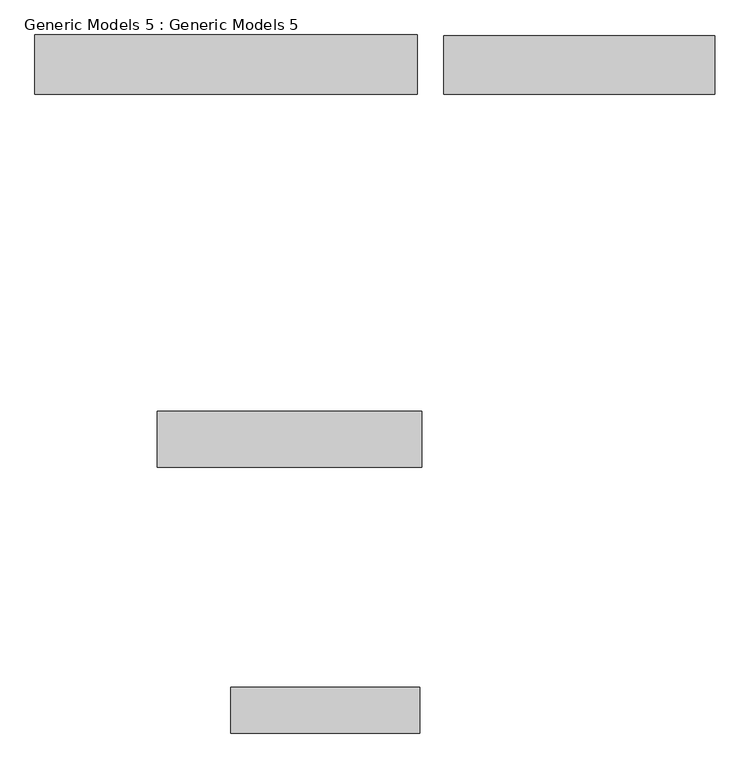
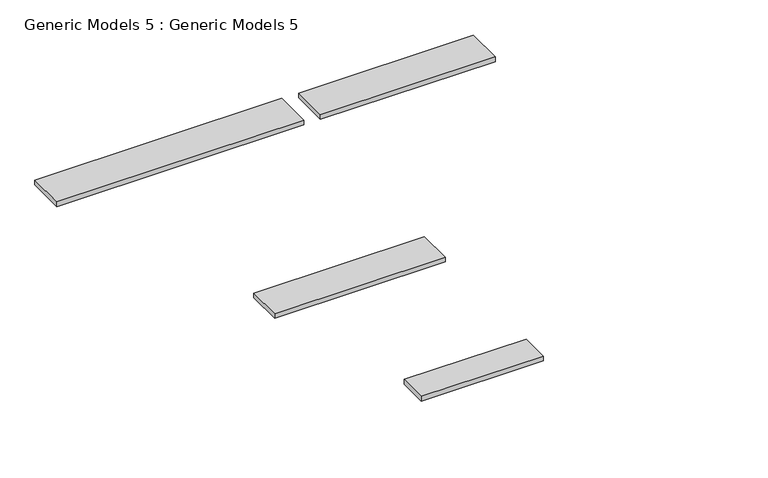
"""IFC4 building model written with IfcOpenShell, lengths in millimetres: proxy geometry, Generic Models 5 : Generic Models 5."""

from ifc_helpers import new_model, si_unit, frame, origin, place, context, project, spatial, polyline, outline, extrude, source, transform, mapped, element, save


def generic_models_5_generic_models_5_efa3826c(model_context):
    return source(origin(), model_context, "Body", "SweptSolid", [
        extrude(outline(polyline([(-40477.34796, 19959.0041063), (-40477.34796, 20415.7418124), (-38591.39796, 20415.7418124), (-38591.39796, 19959.0041063), (-40477.34796, 19959.0041063)])), frame((0.0, 0.0, 1219.2), z_axis=(0.0, 0.0, 1.0), x_axis=(1.0, 0.0, 0.0)), (0.0, 0.0, 1.0), 76.2),
        extrude(outline(polyline([(-41213.94796, 22613.3041063), (-41213.94796, 23172.1041063), (-38572.34796, 23172.1041063), (-38572.34796, 22613.3041063), (-41213.94796, 22613.3041063)])), frame((0.0, 0.0, 1219.2), z_axis=(0.0, 0.0, 1.0), x_axis=(1.0, 0.0, 0.0)), (0.0, 0.0, 1.0), 76.2),
        extrude(outline(polyline([(-42433.14796, 26924.8648243), (-38616.79796, 26924.8648243), (-38616.79796, 26334.3148243), (-42433.14796, 26334.3148243), (-42433.14796, 26924.8648243)])), frame((0.0, 0.0, 1219.2), z_axis=(0.0, 0.0, 1.0), x_axis=(1.0, 0.0, 0.0)), (0.0, 0.0, 1.0), 76.2),
        extrude(outline(polyline([(-35651.34796, 26918.5148243), (-35651.34796, 26332.6177674), (-38356.44796, 26332.6177674), (-38356.44796, 26918.5148243), (-35651.34796, 26918.5148243)])), frame((0.0, 0.0, 1219.2), z_axis=(0.0, 0.0, 1.0), x_axis=(1.0, 0.0, 0.0)), (0.0, 0.0, 1.0), 76.2),
    ])


if __name__ == "__main__":
    model = new_model("IFC4")
    model_context = context("Model", 3, world=origin())
    ifc_project = project(units=[si_unit("LENGTHUNIT", "METRE", prefix="MILLI")], contexts=[model_context])
    site = spatial("IfcSite", under=ifc_project)
    building = spatial("IfcBuilding", under=site)
    placement = place(None, origin())
    generic_models_5_generic_models_5_shape = generic_models_5_generic_models_5_efa3826c(model_context)
    element("IfcBuildingElementProxy", 1, Name="Generic Models 5 : Generic Models 5", ObjectType="Generic Models 5 : Generic Models 5", at=placement, inside=building, context=model_context, shape_type="MappedRepresentation", body=[
        mapped(generic_models_5_generic_models_5_shape, transform((0.0, 0.0, 0.0), x_axis=(1.0, 0.0, 0.0), y_axis=(0.0, 1.0, 0.0), z_axis=(0.0, 0.0, 1.0))),
    ])
    save(model, "model.ifc")
